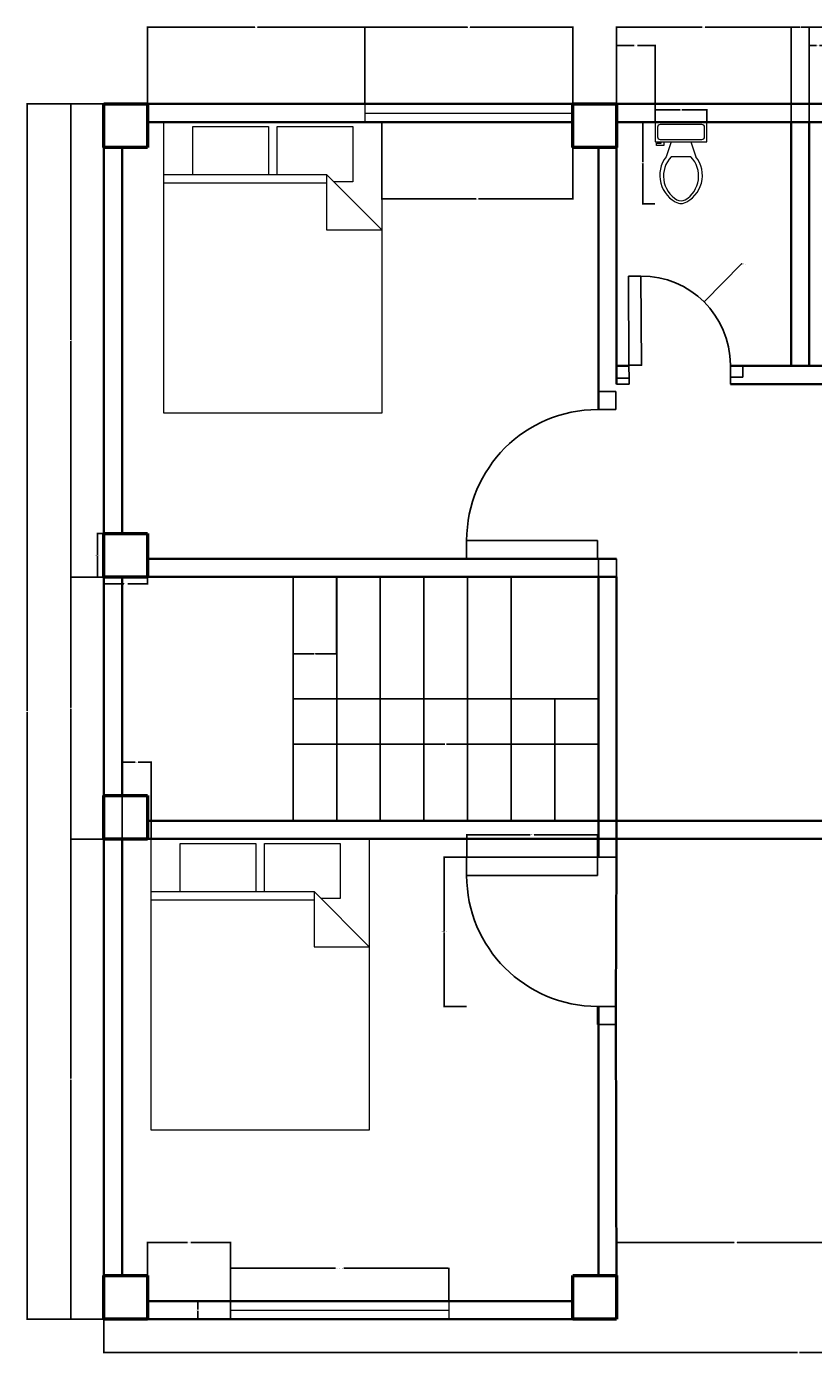
# Model space of a CAD drawing. Units: inches. Extents: x 2082 to 2506, y 790 to 1201.
# Tile 1 of 3: x 2082 to 2298, y 836 to 1201. Entities that reach past the tile are written whole.
import ezdxf

# ---------------------------------------------------------------- set-up
doc = ezdxf.new("R2010")
doc.units = ezdxf.units.IN
for name, color, linetype, lineweight in [('A-ANNO-DIMS', 2, 'Continuous', 18), ('A-COLS', 7, 'Continuous', 50), ('A-DOOR', 3, 'Continuous', 25), ('A-FLOR-FIXT', 9, 'Continuous', 18), ('A-FLOR-STRS', 2, 'Continuous', 25), ('A-FURN', 8, 'Continuous', 18), ('A-GLAZ', 4, 'Continuous', 18), ('A-WALL', 7, 'Continuous', 35)]:
    doc.layers.add(name, color=color, linetype=linetype, lineweight=lineweight)
doc.styles.get("Standard").update_dxf_attribs({"font": 'arial.ttf'})
doc.dimstyles.get("Standard").update_dxf_attribs({"dimtxt": 0.18, "dimasz": 0.18, "dimexe": 0.18, "dimexo": 0.0625, "dimgap": 0.09, "dimtad": 0, "dimtih": 1, "dimtoh": 1, "dimdec": 4, "dimzin": 0, "dimdsep": 46, "dimlunit": 4, "dimtxsty": 'Standard', "dimcen": 0.09, "dimadec": 0, "dimazin": 0, "dimtfac": 1, "dimtdec": 4, "dimtofl": 0, "dimtmove": 0, "dimatfit": 3, "dimfxl": 1, "dimtolj": 1, "dimtzin": 0, "dimarcsym": 0})

# ---------------------------------------------------------------- blocks, each defined once
blk = doc.blocks.new('Toilet - top')
for p, q in [((9.5, -6), (9.5, -2)), ((-10, -8.5), (-8, -8.5)), ((-10, -9.5), (-10, -8.5)), ((-7, -9.5), (-10, -9.5)), ((-8, -8.5), (-8, -8)), ((-7, -8), (-7, -9.5)), ((-4, -8), (-6, -14)), ((4, -8), (6, -14)), ((4, -14), (-4, -14))]:
    blk.add_line(p, q)
blk.add_lwpolyline([(10.5, -8), (10.5, 0), (-10.5, 0), (-10.5, -8)], close=True)
for points in [[(-9.5, -2), (-9.5, -6)], [(8.5, -1), (-8.5, -1)], [(-8.5, -7), (8.5, -7)]]:
    blk.add_lwpolyline(points)
for centre, radius, start, end in [((-8.62, -1.88), 0.884, 81.8699, 188.1301), ((8.62, -1.88), 0.884, 351.8699, 98.1301), ((-8.62, -6.12), 0.884, 171.8699, 278.1301), ((8.62, -6.12), 0.884, 261.8699, 8.1301), ((3.52, -21.58), 12.17, 141.4691, 247.9714), ((4.2, -21.82), 11.33, 136.3677, 238.9468), ((-3.52, -21.58), 12.17, 292.0284, 38.5307), ((-4.2, -21.82), 11.33, 301.053, 43.6321), ((0, -27.88), 4, 245.7318, 294.2682), ((0, -29), 4, 254.8605, 285.1395)]:
    blk.add_arc(centre, radius, start, end)
blk = doc.blocks.new('Bed - Queen')
for p, q in [((0, -80.00003), (0, 0)), ((0, 0), (59.99999, 0)), ((59.99999, 0), (59.99999, -80.00003)), ((7.99999, -1.2), (28.79998, -1.2)), ((7.99999, -14.4), (7.99999, -1.2)), ((28.79998, -1.2), (28.79998, -14.4)), ((31.19999, -1.2), (51.99999, -1.2)), ((31.19999, -14.4), (31.19999, -1.2)), ((51.99999, -1.2), (51.99999, -16.4)), ((0, -14.4), (44.8, -14.4)), ((59.99999, -29.6), (44.8, -14.4)), ((44.8, -14.4), (44.8, -29.6)), ((44.8, -16.8), (0, -16.8)), ((51.99999, -16.4), (46.79936, -16.4)), ((44.8, -29.6), (59.99999, -29.6)), ((59.99999, -80.00003), (0, -80.00003))]:
    blk.add_line(p, q)
blk = doc.blocks.new('DOOR-SWING-36IN')
for p, q in [((0, 0), (0, 5)), ((0, 5), (36, 5)), ((36, 5), (36, 0)), ((36, 0), (0, 0))]:
    blk.add_line(p, q)
blk.add_arc((0, 5), 36, 0, 90)
blk = doc.blocks.new('WIN-60IN')
for p, q in [((0, 5), (12, 5)), ((0, 5), (0, 0)), ((12, 5), (60, 5)), ((60, 5), (60, 0)), ((0, 2.5), (60, 2.5)), ((0, 0), (60, 0))]:
    blk.add_line(p, q)
blk = doc.blocks.new('COL-12X12IN')
for p, q in [((0, 12), (12, 12)), ((0, 0), (0, 12)), ((12, 12), (12, 0)), ((12, 0), (0, 0))]:
    blk.add_line(p, q)
blk = doc.blocks.new('*D8')
at = {"layer": 'A-ANNO-DIMS', "color": 0, "lineweight": -2, "transparency": 16777216}
for p, q in [((2102.86, 1061.45), (2100.94, 1061.45)), ((2101.12, 1061.27), (2101.12, 1055.63)), ((2101.12, 1049.63), (2101.12, 1055.27)), ((2102.86, 1049.45), (2100.94, 1049.45))]:
    blk.add_line(p, q, dxfattribs=at)
at = {"layer": 'A-ANNO-DIMS', "color": 0, "transparency": 16777216}
for points in [[(2101.09, 1061.27), (2101.15, 1061.27), (2101.12, 1061.45)], [(2101.09, 1049.63), (2101.15, 1049.63), (2101.12, 1049.45)]]:
    blk.add_solid(points, dxfattribs=at)
at = {"layer": 'Defpoints', "color": 0, "transparency": 16777216}
for p in [(2101.12, 1061.45), (2102.92, 1061.45), (2102.92, 1049.45)]:
    blk.add_point(p, dxfattribs=at)
at = {"layer": 'A-ANNO-DIMS', "color": 0, "transparency": 16777216, "insert": (2101.12, 1055.45), "char_height": 0.18, "attachment_point": 5}
blk.add_mtext('\\A1;COLUMN 12 TYP.', dxfattribs=at)
blk = doc.blocks.new('*D9')
at = {"layer": 'A-ANNO-DIMS', "color": 0, "lineweight": -2, "transparency": 16777216}
for p, q in [((2102.92, 1049.39), (2102.92, 1047.47)), ((2103.1, 1047.65), (2108.4, 1047.65)), ((2114.74, 1047.65), (2109.44, 1047.65)), ((2114.92, 1049.39), (2114.92, 1047.47))]:
    blk.add_line(p, q, dxfattribs=at)
at = {"layer": 'A-ANNO-DIMS', "color": 0, "transparency": 16777216}
for points in [[(2103.1, 1047.68), (2103.1, 1047.62), (2102.92, 1047.65)], [(2114.74, 1047.68), (2114.74, 1047.62), (2114.92, 1047.65)]]:
    blk.add_solid(points, dxfattribs=at)
at = {"layer": 'Defpoints', "color": 0, "transparency": 16777216}
for p in [(2102.92, 1049.45), (2102.92, 1047.65), (2114.92, 1049.45)]:
    blk.add_point(p, dxfattribs=at)
at = {"layer": 'A-ANNO-DIMS', "color": 0, "transparency": 16777216, "insert": (2108.92, 1047.65), "char_height": 0.18, "attachment_point": 5}
blk.add_mtext('\\A1;12 TYP.', dxfattribs=at)
blk = doc.blocks.new('*D12')
at = {"layer": 'A-ANNO-DIMS', "color": 0, "lineweight": -2, "transparency": 16777216}
for p, q in [((2137.75, 850.56), (2137.75, 859.68)), ((2137.93, 859.5), (2166.63, 859.5)), ((2197.57, 859.5), (2168.87, 859.5)), ((2197.75, 850.56), (2197.75, 859.68))]:
    blk.add_line(p, q, dxfattribs=at)
at = {"layer": 'A-ANNO-DIMS', "color": 0, "transparency": 16777216}
for points in [[(2137.93, 859.53), (2137.93, 859.47), (2137.75, 859.5)], [(2197.57, 859.53), (2197.57, 859.47), (2197.75, 859.5)]]:
    blk.add_solid(points, dxfattribs=at)
at = {"layer": 'Defpoints', "color": 0, "transparency": 16777216}
for p in [(2197.75, 859.5), (2137.75, 850.5), (2197.75, 850.5)]:
    blk.add_point(p, dxfattribs=at)
at = {"layer": 'A-ANNO-DIMS', "color": 0, "transparency": 16777216, "insert": (2167.75, 859.5), "char_height": 0.18, "attachment_point": 5}
blk.add_mtext('\\A1;WINDOW 60 TYP.', dxfattribs=at)
blk = doc.blocks.new('*D13')
at = {"layer": 'A-ANNO-DIMS', "color": 0, "lineweight": -2, "transparency": 16777216}
for p, q in [((2137.69, 850.5), (2128.57, 850.5)), ((2128.75, 850.32), (2128.75, 848.18)), ((2128.75, 845.68), (2128.75, 847.82)), ((2137.69, 845.5), (2128.57, 845.5))]:
    blk.add_line(p, q, dxfattribs=at)
at = {"layer": 'A-ANNO-DIMS', "color": 0, "transparency": 16777216}
for points in [[(2128.72, 850.32), (2128.78, 850.32), (2128.75, 850.5)], [(2128.72, 845.68), (2128.78, 845.68), (2128.75, 845.5)]]:
    blk.add_solid(points, dxfattribs=at)
at = {"layer": 'Defpoints', "color": 0, "transparency": 16777216}
for p in [(2128.75, 850.5), (2137.75, 850.5), (2137.75, 845.5)]:
    blk.add_point(p, dxfattribs=at)
at = {"layer": 'A-ANNO-DIMS', "color": 0, "transparency": 16777216, "insert": (2128.75, 848), "char_height": 0.18, "attachment_point": 5}
blk.add_mtext('\\A1;5 TYP.', dxfattribs=at)
blk = doc.blocks.new('*D14')
at = {"layer": 'A-ANNO-DIMS', "color": 0, "lineweight": -2, "transparency": 16777216}
for p, q in [((2202.61, 972.5), (2196.35, 972.5)), ((2196.53, 972.32), (2196.53, 952.18)), ((2196.53, 931.68), (2196.53, 951.82)), ((2202.61, 931.5), (2196.35, 931.5))]:
    blk.add_line(p, q, dxfattribs=at)
at = {"layer": 'A-ANNO-DIMS', "color": 0, "transparency": 16777216}
for points in [[(2196.5, 972.32), (2196.56, 972.32), (2196.53, 972.5)], [(2196.5, 931.68), (2196.56, 931.68), (2196.53, 931.5)]]:
    blk.add_solid(points, dxfattribs=at)
at = {"layer": 'Defpoints', "color": 0, "transparency": 16777216}
for p in [(2202.68, 972.5), (2196.53, 931.5), (2202.68, 931.5)]:
    blk.add_point(p, dxfattribs=at)
at = {"layer": 'A-ANNO-DIMS', "color": 0, "transparency": 16777216, "insert": (2196.53, 952), "char_height": 0.18, "attachment_point": 5}
blk.add_mtext('\\A1;DOOR 41 TYP.', dxfattribs=at)
blk = doc.blocks.new('*D15')
at = {"layer": 'A-ANNO-DIMS', "color": 0, "lineweight": -2, "transparency": 16777216}
for p, q in [((2202.68, 972.56), (2202.68, 978.83)), ((2202.86, 978.65), (2220.15, 978.65)), ((2238.5, 978.65), (2221.2, 978.65)), ((2238.68, 972.56), (2238.68, 978.83))]:
    blk.add_line(p, q, dxfattribs=at)
at = {"layer": 'A-ANNO-DIMS', "color": 0, "transparency": 16777216}
for points in [[(2202.86, 978.68), (2202.86, 978.62), (2202.68, 978.65)], [(2238.5, 978.68), (2238.5, 978.62), (2238.68, 978.65)]]:
    blk.add_solid(points, dxfattribs=at)
at = {"layer": 'Defpoints', "color": 0, "transparency": 16777216}
for p in [(2202.68, 978.65), (2202.68, 972.5), (2238.68, 972.5)]:
    blk.add_point(p, dxfattribs=at)
at = {"layer": 'A-ANNO-DIMS', "color": 0, "transparency": 16777216, "insert": (2220.68, 978.65), "char_height": 0.18, "attachment_point": 5}
blk.add_mtext('\\A1;36 TYP.', dxfattribs=at)
blk = doc.blocks.new('*D16')
at = {"layer": 'A-ANNO-DIMS', "color": 0, "lineweight": -2, "transparency": 16777216}
for p, q in [((2254.46, 1174.5), (2250.98, 1174.5)), ((2251.16, 1174.32), (2251.16, 1163.48)), ((2251.16, 1152.27), (2251.16, 1163.11)), ((2254.46, 1152.09), (2250.98, 1152.09))]:
    blk.add_line(p, q, dxfattribs=at)
at = {"layer": 'A-ANNO-DIMS', "color": 0, "transparency": 16777216}
for points in [[(2251.13, 1174.32), (2251.19, 1174.32), (2251.16, 1174.5)], [(2251.13, 1152.27), (2251.19, 1152.27), (2251.16, 1152.09)]]:
    blk.add_solid(points, dxfattribs=at)
at = {"layer": 'Defpoints', "color": 0, "transparency": 16777216}
for p in [(2251.16, 1174.5), (2254.52, 1174.5), (2254.52, 1152.09)]:
    blk.add_point(p, dxfattribs=at)
at = {"layer": 'A-ANNO-DIMS', "color": 0, "transparency": 16777216, "insert": (2251.16, 1163.3), "char_height": 0.18, "attachment_point": 5}
blk.add_mtext('\\A1;WC 22', dxfattribs=at)
blk = doc.blocks.new('*D17')
at = {"layer": 'A-ANNO-DIMS', "color": 0, "lineweight": -2, "transparency": 16777216}
for p, q in [((2254.52, 1174.56), (2254.52, 1178.04)), ((2268.76, 1174.56), (2268.76, 1178.04)), ((2254.7, 1177.86), (2261.43, 1177.86)), ((2268.58, 1177.86), (2261.85, 1177.86))]:
    blk.add_line(p, q, dxfattribs=at)
at = {"layer": 'A-ANNO-DIMS', "color": 0, "transparency": 16777216}
for points in [[(2254.7, 1177.89), (2254.7, 1177.83), (2254.52, 1177.86)], [(2268.58, 1177.89), (2268.58, 1177.83), (2268.76, 1177.86)]]:
    blk.add_solid(points, dxfattribs=at)
at = {"layer": 'Defpoints', "color": 0, "transparency": 16777216}
for p in [(2254.52, 1174.5), (2268.76, 1177.86), (2268.76, 1174.5)]:
    blk.add_point(p, dxfattribs=at)
at = {"layer": 'A-ANNO-DIMS', "color": 0, "transparency": 16777216, "insert": (2261.64, 1177.86), "char_height": 0.18, "attachment_point": 5}
blk.add_mtext('\\A1;14', dxfattribs=at)
blk = doc.blocks.new('*D24')
at = {"layer": 'A-ANNO-DIMS', "color": 0, "lineweight": -2, "transparency": 16777216}
for p, q in [((2102.92, 857.43), (2102.92, 836.21)), ((2484.95, 857.32), (2484.95, 836.1)), ((2103.1, 836.39), (2293.64, 836.34)), ((2484.77, 836.28), (2294.22, 836.34))]:
    blk.add_line(p, q, dxfattribs=at)
at = {"layer": 'A-ANNO-DIMS', "color": 0, "transparency": 16777216}
for points in [[(2103.1, 836.42), (2103.1, 836.36), (2102.92, 836.39)], [(2484.77, 836.31), (2484.77, 836.25), (2484.95, 836.28)]]:
    blk.add_solid(points, dxfattribs=at)
at = {"layer": 'Defpoints', "color": 0, "transparency": 16777216}
for p in [(2102.92, 857.49), (2484.95, 857.38), (2102.92, 836.39)]:
    blk.add_point(p, dxfattribs=at)
at = {"layer": 'A-ANNO-DIMS', "color": 0, "transparency": 16777216, "insert": (2293.93, 836.34), "char_height": 0.18, "attachment_point": 5}
blk.add_mtext('\\A1;382', dxfattribs=at)
blk = doc.blocks.new('*D25')
at = {"layer": 'A-ANNO-DIMS', "color": 0, "lineweight": -2, "transparency": 16777216}
for p, q in [((2102.86, 1179.5), (2081.64, 1179.5)), ((2081.82, 1179.32), (2081.82, 1012.68)), ((2081.82, 845.67), (2081.82, 1012.31)), ((2102.86, 845.49), (2081.64, 845.49))]:
    blk.add_line(p, q, dxfattribs=at)
at = {"layer": 'A-ANNO-DIMS', "color": 0, "transparency": 16777216}
for points in [[(2081.79, 1179.32), (2081.85, 1179.32), (2081.82, 1179.5)], [(2081.79, 845.67), (2081.85, 845.67), (2081.82, 845.49)]]:
    blk.add_solid(points, dxfattribs=at)
at = {"layer": 'Defpoints', "color": 0, "transparency": 16777216}
for p in [(2081.82, 1179.5), (2102.92, 1179.5), (2102.92, 845.49)]:
    blk.add_point(p, dxfattribs=at)
at = {"layer": 'A-ANNO-DIMS', "color": 0, "transparency": 16777216, "insert": (2081.82, 1012.5), "char_height": 0.18, "attachment_point": 5}
blk.add_mtext('\\A1;334', dxfattribs=at)
blk = doc.blocks.new('*D26')
at = {"layer": 'A-ANNO-DIMS', "color": 0, "lineweight": -2, "transparency": 16777216}
for p, q in [((2114.86, 977.48), (2093.64, 977.48)), ((2093.82, 977.3), (2093.82, 911.67)), ((2093.82, 845.67), (2093.82, 911.3)), ((2114.86, 845.49), (2093.64, 845.49))]:
    blk.add_line(p, q, dxfattribs=at)
at = {"layer": 'A-ANNO-DIMS', "color": 0, "transparency": 16777216}
for points in [[(2093.79, 977.3), (2093.85, 977.3), (2093.82, 977.48)], [(2093.79, 845.67), (2093.85, 845.67), (2093.82, 845.49)]]:
    blk.add_solid(points, dxfattribs=at)
at = {"layer": 'Defpoints', "color": 0, "transparency": 16777216}
for p in [(2093.82, 977.48), (2114.92, 977.48), (2114.92, 845.49)]:
    blk.add_point(p, dxfattribs=at)
at = {"layer": 'A-ANNO-DIMS', "color": 0, "transparency": 16777216, "insert": (2093.82, 911.49), "char_height": 0.18, "attachment_point": 5}
blk.add_mtext('\\A1;132', dxfattribs=at)
blk = doc.blocks.new('*D27')
at = {"layer": 'A-ANNO-DIMS', "color": 0, "lineweight": -2, "transparency": 16777216}
for p, q in [((2114.86, 1049.45), (2093.64, 1049.45)), ((2093.82, 1049.27), (2093.82, 1013.65)), ((2093.82, 977.66), (2093.82, 1013.28)), ((2114.86, 977.48), (2093.64, 977.48))]:
    blk.add_line(p, q, dxfattribs=at)
at = {"layer": 'A-ANNO-DIMS', "color": 0, "transparency": 16777216}
for points in [[(2093.79, 1049.27), (2093.85, 1049.27), (2093.82, 1049.45)], [(2093.79, 977.66), (2093.85, 977.66), (2093.82, 977.48)]]:
    blk.add_solid(points, dxfattribs=at)
at = {"layer": 'Defpoints', "color": 0, "transparency": 16777216}
for p in [(2093.82, 1049.45), (2114.92, 1049.45), (2114.92, 977.48)]:
    blk.add_point(p, dxfattribs=at)
at = {"layer": 'A-ANNO-DIMS', "color": 0, "transparency": 16777216, "insert": (2093.82, 1013.47), "char_height": 0.18, "attachment_point": 5}
blk.add_mtext('\\A1;71.97', dxfattribs=at)
blk = doc.blocks.new('*D28')
at = {"layer": 'A-ANNO-DIMS', "color": 0, "lineweight": -2, "transparency": 16777216}
for p, q in [((2114.86, 1179.5), (2093.64, 1179.5)), ((2093.82, 1179.32), (2093.82, 1114.66)), ((2093.82, 1049.63), (2093.82, 1114.29)), ((2114.86, 1049.45), (2093.64, 1049.45))]:
    blk.add_line(p, q, dxfattribs=at)
at = {"layer": 'A-ANNO-DIMS', "color": 0, "transparency": 16777216}
for points in [[(2093.79, 1179.32), (2093.85, 1179.32), (2093.82, 1179.5)], [(2093.79, 1049.63), (2093.85, 1049.63), (2093.82, 1049.45)]]:
    blk.add_solid(points, dxfattribs=at)
at = {"layer": 'Defpoints', "color": 0, "transparency": 16777216}
for p in [(2093.82, 1179.5), (2114.92, 1179.5), (2114.92, 1049.45)]:
    blk.add_point(p, dxfattribs=at)
at = {"layer": 'A-ANNO-DIMS', "color": 0, "transparency": 16777216, "insert": (2093.82, 1114.47), "char_height": 0.18, "attachment_point": 5}
blk.add_mtext('\\A1;130.05', dxfattribs=at)
blk = doc.blocks.new('*D29')
at = {"layer": 'A-ANNO-DIMS', "color": 0, "lineweight": -2, "transparency": 16777216}
for p, q in [((2114.92, 1179.56), (2114.92, 1200.78)), ((2115.1, 1200.6), (2144.4, 1200.6)), ((2174.49, 1200.6), (2145.19, 1200.6)), ((2174.67, 1179.56), (2174.67, 1200.78))]:
    blk.add_line(p, q, dxfattribs=at)
at = {"layer": 'A-ANNO-DIMS', "color": 0, "transparency": 16777216}
for points in [[(2115.1, 1200.63), (2115.1, 1200.57), (2114.92, 1200.6)], [(2174.49, 1200.63), (2174.49, 1200.57), (2174.67, 1200.6)]]:
    blk.add_solid(points, dxfattribs=at)
at = {"layer": 'Defpoints', "color": 0, "transparency": 16777216}
for p in [(2174.67, 1200.6), (2114.92, 1179.5), (2174.67, 1179.5)]:
    blk.add_point(p, dxfattribs=at)
at = {"layer": 'A-ANNO-DIMS', "color": 0, "transparency": 16777216, "insert": (2144.8, 1200.6), "char_height": 0.18, "attachment_point": 5}
blk.add_mtext('\\A1;59.75', dxfattribs=at)
blk = doc.blocks.new('*D30')
at = {"layer": 'A-ANNO-DIMS', "color": 0, "lineweight": -2, "transparency": 16777216}
for p, q in [((2174.67, 1179.56), (2174.67, 1200.78)), ((2174.85, 1200.6), (2202.87, 1200.6)), ((2231.68, 1200.6), (2203.66, 1200.6)), ((2231.86, 1179.56), (2231.86, 1200.78))]:
    blk.add_line(p, q, dxfattribs=at)
at = {"layer": 'A-ANNO-DIMS', "color": 0, "transparency": 16777216}
for points in [[(2174.85, 1200.63), (2174.85, 1200.57), (2174.67, 1200.6)], [(2231.68, 1200.63), (2231.68, 1200.57), (2231.86, 1200.6)]]:
    blk.add_solid(points, dxfattribs=at)
at = {"layer": 'Defpoints', "color": 0, "transparency": 16777216}
for p in [(2231.86, 1200.6), (2174.67, 1179.5), (2231.86, 1179.5)]:
    blk.add_point(p, dxfattribs=at)
at = {"layer": 'A-ANNO-DIMS', "color": 0, "transparency": 16777216, "insert": (2203.26, 1200.6), "char_height": 0.18, "attachment_point": 5}
blk.add_mtext('\\A1;57.18', dxfattribs=at)
blk = doc.blocks.new('*D31')
at = {"layer": 'A-ANNO-DIMS', "color": 0, "lineweight": -2, "transparency": 16777216}
for p, q in [((2243.86, 1174.56), (2243.86, 1200.78)), ((2244.04, 1200.6), (2267.49, 1200.6)), ((2291.74, 1200.6), (2268.29, 1200.6)), ((2291.92, 1174.56), (2291.92, 1200.78))]:
    blk.add_line(p, q, dxfattribs=at)
at = {"layer": 'A-ANNO-DIMS', "color": 0, "transparency": 16777216}
for points in [[(2244.04, 1200.63), (2244.04, 1200.57), (2243.86, 1200.6)], [(2291.74, 1200.63), (2291.74, 1200.57), (2291.92, 1200.6)]]:
    blk.add_solid(points, dxfattribs=at)
at = {"layer": 'Defpoints', "color": 0, "transparency": 16777216}
for p in [(2291.92, 1200.6), (2243.86, 1174.5), (2291.92, 1174.5)]:
    blk.add_point(p, dxfattribs=at)
at = {"layer": 'A-ANNO-DIMS', "color": 0, "transparency": 16777216, "insert": (2267.89, 1200.6), "char_height": 0.18, "attachment_point": 5}
blk.add_mtext('\\A1;48.07', dxfattribs=at)
blk = doc.blocks.new('*D32')
at = {"layer": 'A-ANNO-DIMS', "color": 0, "lineweight": -2, "transparency": 16777216}
for p, q in [((2291.92, 1174.56), (2291.92, 1200.78)), ((2292.1, 1200.6), (2294.27, 1200.6)), ((2296.74, 1200.6), (2294.57, 1200.6)), ((2296.92, 1174.56), (2296.92, 1200.78))]:
    blk.add_line(p, q, dxfattribs=at)
at = {"layer": 'A-ANNO-DIMS', "color": 0, "transparency": 16777216}
for points in [[(2292.1, 1200.63), (2292.1, 1200.57), (2291.92, 1200.6)], [(2296.74, 1200.63), (2296.74, 1200.57), (2296.92, 1200.6)]]:
    blk.add_solid(points, dxfattribs=at)
at = {"layer": 'Defpoints', "color": 0, "transparency": 16777216}
for p in [(2296.92, 1200.6), (2291.92, 1174.5), (2296.92, 1174.5)]:
    blk.add_point(p, dxfattribs=at)
at = {"layer": 'A-ANNO-DIMS', "color": 0, "transparency": 16777216, "insert": (2294.42, 1200.6), "char_height": 0.18, "attachment_point": 5}
blk.add_mtext('\\A1;5', dxfattribs=at)
blk = doc.blocks.new('*D33')
at = {"layer": 'A-ANNO-DIMS', "color": 0, "lineweight": -2, "transparency": 16777216}
for p, q in [((2296.92, 1174.56), (2296.92, 1200.78)), ((2297.1, 1200.6), (2317.7, 1200.6)), ((2338.74, 1200.6), (2318.15, 1200.6)), ((2338.92, 1174.56), (2338.92, 1200.78))]:
    blk.add_line(p, q, dxfattribs=at)
at = {"layer": 'A-ANNO-DIMS', "color": 0, "transparency": 16777216}
for points in [[(2297.1, 1200.63), (2297.1, 1200.57), (2296.92, 1200.6)], [(2338.74, 1200.63), (2338.74, 1200.57), (2338.92, 1200.6)]]:
    blk.add_solid(points, dxfattribs=at)
at = {"layer": 'Defpoints', "color": 0, "transparency": 16777216}
for p in [(2338.92, 1200.6), (2296.92, 1174.5), (2338.92, 1174.5)]:
    blk.add_point(p, dxfattribs=at)
at = {"layer": 'A-ANNO-DIMS', "color": 0, "transparency": 16777216, "insert": (2317.92, 1200.6), "char_height": 0.18, "attachment_point": 5}
blk.add_mtext('\\A1;42', dxfattribs=at)
blk = doc.blocks.new('*D39')
at = {"layer": 'A-ANNO-DIMS', "color": 0, "lineweight": -2, "transparency": 16777216}
for p, q in [((2154.92, 982.56), (2154.92, 1003.78)), ((2155.1, 1003.6), (2196.7, 1003.6)), ((2238.74, 1003.6), (2197.14, 1003.6)), ((2238.92, 982.56), (2238.92, 1003.78))]:
    blk.add_line(p, q, dxfattribs=at)
at = {"layer": 'A-ANNO-DIMS', "color": 0, "transparency": 16777216}
for points in [[(2155.1, 1003.63), (2155.1, 1003.57), (2154.92, 1003.6)], [(2238.74, 1003.63), (2238.74, 1003.57), (2238.92, 1003.6)]]:
    blk.add_solid(points, dxfattribs=at)
at = {"layer": 'Defpoints', "color": 0, "transparency": 16777216}
for p in [(2238.92, 1003.6), (2154.92, 982.5), (2238.92, 982.5)]:
    blk.add_point(p, dxfattribs=at)
at = {"layer": 'A-ANNO-DIMS', "color": 0, "transparency": 16777216, "insert": (2196.92, 1003.6), "char_height": 0.18, "attachment_point": 5}
blk.add_mtext('\\A1;84', dxfattribs=at)
blk = doc.blocks.new('*D40')
at = {"layer": 'A-ANNO-DIMS', "color": 0, "lineweight": -2, "transparency": 16777216}
for p, q in [((2154.92, 1049.44), (2154.92, 1028.22)), ((2166.92, 1049.44), (2166.92, 1028.22)), ((2155.1, 1028.4), (2160.71, 1028.4)), ((2166.74, 1028.4), (2161.13, 1028.4))]:
    blk.add_line(p, q, dxfattribs=at)
at = {"layer": 'A-ANNO-DIMS', "color": 0, "transparency": 16777216}
for points in [[(2155.1, 1028.43), (2155.1, 1028.37), (2154.92, 1028.4)], [(2166.74, 1028.43), (2166.74, 1028.37), (2166.92, 1028.4)]]:
    blk.add_solid(points, dxfattribs=at)
at = {"layer": 'Defpoints', "color": 0, "transparency": 16777216}
for p in [(2154.92, 1049.5), (2166.92, 1049.5), (2154.92, 1028.4)]:
    blk.add_point(p, dxfattribs=at)
at = {"layer": 'A-ANNO-DIMS', "color": 0, "transparency": 16777216, "insert": (2160.92, 1028.4), "char_height": 0.18, "attachment_point": 5}
blk.add_mtext('\\A1;12', dxfattribs=at)
blk = doc.blocks.new('*D41')
at = {"layer": 'A-ANNO-DIMS', "color": 0, "lineweight": -2, "transparency": 16777216}
for p, q in [((2243.9, 845.56), (2243.9, 866.78)), ((2244.08, 866.6), (2276.28, 866.6)), ((2309.24, 866.6), (2277.04, 866.6)), ((2309.42, 845.56), (2309.42, 866.78))]:
    blk.add_line(p, q, dxfattribs=at)
at = {"layer": 'A-ANNO-DIMS', "color": 0, "transparency": 16777216}
for points in [[(2244.08, 866.63), (2244.08, 866.57), (2243.9, 866.6)], [(2309.24, 866.63), (2309.24, 866.57), (2309.42, 866.6)]]:
    blk.add_solid(points, dxfattribs=at)
at = {"layer": 'Defpoints', "color": 0, "transparency": 16777216}
for p in [(2309.42, 866.6), (2243.9, 845.5), (2309.42, 845.5)]:
    blk.add_point(p, dxfattribs=at)
at = {"layer": 'A-ANNO-DIMS', "color": 0, "transparency": 16777216, "insert": (2276.66, 866.6), "char_height": 0.18, "attachment_point": 5}
blk.add_mtext('\\A1;65.51', dxfattribs=at)
blk = doc.blocks.new('*D42')
at = {"layer": 'A-ANNO-DIMS', "color": 0, "lineweight": -2, "transparency": 16777216}
for p, q in [((2114.92, 845.55), (2114.92, 866.77)), ((2115.1, 866.59), (2125.86, 866.6)), ((2137.56, 866.6), (2126.8, 866.6)), ((2137.75, 845.56), (2137.74, 866.78))]:
    blk.add_line(p, q, dxfattribs=at)
at = {"layer": 'A-ANNO-DIMS', "color": 0, "transparency": 16777216}
for points in [[(2115.1, 866.62), (2115.1, 866.56), (2114.92, 866.59)], [(2137.56, 866.63), (2137.56, 866.57), (2137.74, 866.6)]]:
    blk.add_solid(points, dxfattribs=at)
at = {"layer": 'Defpoints', "color": 0, "transparency": 16777216}
for p in [(2137.74, 866.6), (2114.92, 845.49), (2137.75, 845.5)]:
    blk.add_point(p, dxfattribs=at)
at = {"layer": 'A-ANNO-DIMS', "color": 0, "transparency": 16777216, "insert": (2126.33, 866.6), "char_height": 0.18, "attachment_point": 5}
blk.add_mtext('\\A1;22.825', dxfattribs=at)
blk = doc.blocks.new('*D49')
at = {"layer": 'A-ANNO-DIMS', "color": 0, "lineweight": -2, "transparency": 16777216}
for p, q in [((2179.35, 1174.44), (2179.35, 1153.22)), ((2231.86, 1174.44), (2231.86, 1153.22)), ((2179.53, 1153.4), (2205.28, 1153.4)), ((2231.68, 1153.4), (2205.93, 1153.4))]:
    blk.add_line(p, q, dxfattribs=at)
at = {"layer": 'A-ANNO-DIMS', "color": 0, "transparency": 16777216}
for points in [[(2179.53, 1153.43), (2179.53, 1153.37), (2179.35, 1153.4)], [(2231.68, 1153.43), (2231.68, 1153.37), (2231.86, 1153.4)]]:
    blk.add_solid(points, dxfattribs=at)
at = {"layer": 'Defpoints', "color": 0, "transparency": 16777216}
for p in [(2179.35, 1174.5), (2231.86, 1174.5), (2179.35, 1153.4)]:
    blk.add_point(p, dxfattribs=at)
at = {"layer": 'A-ANNO-DIMS', "color": 0, "transparency": 16777216, "insert": (2205.6, 1153.4), "char_height": 0.18, "attachment_point": 5}
blk.add_mtext('\\A1;52.5', dxfattribs=at)
blk = doc.blocks.new('*D51')
at = {"layer": 'A-ANNO-DIMS', "color": 0, "lineweight": -2, "transparency": 16777216}
for p, q in [((2107.92, 977.56), (2107.92, 998.78)), ((2108.1, 998.6), (2111.52, 998.6)), ((2115.73, 998.6), (2112.31, 998.6)), ((2115.91, 977.56), (2115.91, 998.78))]:
    blk.add_line(p, q, dxfattribs=at)
at = {"layer": 'A-ANNO-DIMS', "color": 0, "transparency": 16777216}
for points in [[(2108.1, 998.63), (2108.1, 998.57), (2107.92, 998.6)], [(2115.73, 998.63), (2115.73, 998.57), (2115.91, 998.6)]]:
    blk.add_solid(points, dxfattribs=at)
at = {"layer": 'Defpoints', "color": 0, "transparency": 16777216}
for p in [(2115.91, 998.6), (2107.92, 977.5), (2115.91, 977.5)]:
    blk.add_point(p, dxfattribs=at)
at = {"layer": 'A-ANNO-DIMS', "color": 0, "transparency": 16777216, "insert": (2111.91, 998.6), "char_height": 0.18, "attachment_point": 5}
blk.add_mtext('\\A1;7.982', dxfattribs=at)
blk = doc.blocks.new('*D52')
at = {"layer": 'A-ANNO-DIMS', "color": 0, "lineweight": -2, "transparency": 16777216}
for p, q in [((2243.86, 1174.56), (2243.86, 1195.78)), ((2244.04, 1195.6), (2248.73, 1195.6)), ((2254.34, 1195.6), (2249.64, 1195.6)), ((2254.52, 1174.56), (2254.52, 1195.78))]:
    blk.add_line(p, q, dxfattribs=at)
at = {"layer": 'A-ANNO-DIMS', "color": 0, "transparency": 16777216}
for points in [[(2244.04, 1195.63), (2244.04, 1195.57), (2243.86, 1195.6)], [(2254.34, 1195.63), (2254.34, 1195.57), (2254.52, 1195.6)]]:
    blk.add_solid(points, dxfattribs=at)
at = {"layer": 'Defpoints', "color": 0, "transparency": 16777216}
for p in [(2254.52, 1195.6), (2243.86, 1174.5), (2254.52, 1174.5)]:
    blk.add_point(p, dxfattribs=at)
at = {"layer": 'A-ANNO-DIMS', "color": 0, "transparency": 16777216, "insert": (2249.19, 1195.6), "char_height": 0.18, "attachment_point": 5}
blk.add_mtext('\\A1;10.666', dxfattribs=at)
blk = doc.blocks.new('*D53')
at = {"layer": 'A-ANNO-DIMS', "color": 0, "lineweight": -2, "transparency": 16777216}
for p, q in [((2296.92, 1174.56), (2296.92, 1195.78)), ((2297.1, 1195.6), (2298.93, 1195.6)), ((2301.55, 1195.6), (2299.72, 1195.6)), ((2301.73, 1174.56), (2301.73, 1195.78))]:
    blk.add_line(p, q, dxfattribs=at)
at = {"layer": 'A-ANNO-DIMS', "color": 0, "transparency": 16777216}
for points in [[(2297.1, 1195.63), (2297.1, 1195.57), (2296.92, 1195.6)], [(2301.55, 1195.63), (2301.55, 1195.57), (2301.73, 1195.6)]]:
    blk.add_solid(points, dxfattribs=at)
at = {"layer": 'Defpoints', "color": 0, "transparency": 16777216}
for p in [(2301.73, 1195.6), (2296.92, 1174.5), (2301.73, 1174.5)]:
    blk.add_point(p, dxfattribs=at)
at = {"layer": 'A-ANNO-DIMS', "color": 0, "transparency": 16777216, "insert": (2299.33, 1195.6), "char_height": 0.18, "attachment_point": 5}
blk.add_mtext('\\A1;4.805', dxfattribs=at)
blk = doc.blocks.new('*D56')
at = {"layer": 'A-ANNO-DIMS', "color": 0, "lineweight": -2, "transparency": 16777216}
for p, q in [((2278.3, 1135.55), (2268.09, 1125.23)), ((2278.48, 1135.55), (2278.3, 1135.55)), ((2250.64, 1107.7), (2250.82, 1107.7)), ((2250.73, 1107.61), (2250.73, 1107.79))]:
    blk.add_line(p, q, dxfattribs=at)
at = {"layer": 'A-ANNO-DIMS', "color": 0, "transparency": 16777216}
blk.add_solid([(2268.07, 1125.25), (2268.11, 1125.21), (2267.96, 1125.1)], dxfattribs=at)
at = {"layer": 'Defpoints', "color": 0, "transparency": 16777216}
for p in [(2267.96, 1125.1), (2250.73, 1107.7)]:
    blk.add_point(p, dxfattribs=at)
at = {"layer": 'A-ANNO-DIMS', "color": 0, "transparency": 16777216, "insert": (2279.03, 1135.55), "char_height": 0.18, "attachment_point": 5}
blk.add_mtext('\\A1;R24.494', dxfattribs=at)

msp = doc.modelspace()

# ---------------------------------------------------------------- linework, layer by layer
at = {"layer": 'A-DOOR'}
for p, q in [((2250.6073, 1132.1933), (2247.2054, 1132.1768)), ((2247.2054, 1132.1768), (2247.3247, 1107.6834)), ((2250.7265, 1107.6999), (2250.6073, 1132.1933)), ((2243.9236, 1107.4988), (2247.3255, 1107.5154)), ((2243.9402, 1104.097), (2243.9236, 1107.4988)), ((2247.3247, 1107.6834), (2250.7265, 1107.6999)), ((2247.3255, 1107.5154), (2247.3421, 1104.1135)), ((2275.2365, 1104.4173), (2275.22, 1107.8192)), ((2278.6235, 1107.4988), (2278.6384, 1104.4339)), ((2247.3498, 1102.5155), (2243.9236, 1102.4988)), ((2247.3421, 1104.1135), (2243.9402, 1104.097)), ((2247.3421, 1104.1135), (2247.3498, 1102.5155)), ((2278.6384, 1104.4339), (2275.2365, 1104.4173)), ((2275.2365, 1104.4173), (2275.2459, 1102.4988)), ((2238.9236, 1100.4988), (2243.6767, 1100.4988)), ((2243.6767, 1100.4988), (2243.6767, 1095.4988)), ((2243.6767, 1095.4988), (2238.6767, 1095.4988)), ((2238.9236, 1049.4988), (2238.9236, 1054.4988)), ((2238.9236, 1054.4988), (2243.9236, 1054.4988)), ((2238.9236, 1054.4988), (2238.9236, 1049.4988)), ((2243.8994, 1054.4988), (2243.9236, 1049.4988)), ((2243.9236, 1054.4988), (2243.9236, 1049.4988)), ((2243.9236, 1049.4988), (2238.9236, 1049.4988)), ((2243.9236, 977.4988), (2238.9236, 977.4988)), ((2243.9236, 977.4988), (2238.9236, 977.4988)), ((2238.9236, 977.4988), (2238.9236, 972.4988)), ((2243.8994, 972.4988), (2243.9236, 977.4988)), ((2238.9236, 972.4988), (2243.9236, 972.4988)), ((2243.6767, 931.4988), (2238.6767, 931.4988)), ((2238.6767, 931.4988), (2238.6767, 926.4988)), ((2243.6767, 926.4988), (2243.6767, 931.4988)), ((2238.6767, 926.4988), (2243.6767, 926.4988))]:
    msp.add_line(p, q, dxfattribs=at)
msp.add_arc((2250.7265, 1107.6999), 24.4937, 0.27894, 90.27894, dxfattribs=at)
at = {"layer": 'A-FLOR-STRS'}
for p, q in [((2154.9236, 1049.4988), (2154.9236, 982.4988)), ((2166.9236, 1049.4988), (2166.9236, 982.4988)), ((2178.9236, 1049.4988), (2178.9236, 982.4988)), ((2190.9236, 1049.4988), (2190.9236, 982.4988)), ((2202.9236, 1049.4988), (2202.9236, 982.4988)), ((2214.9236, 1049.4988), (2214.9236, 982.4988)), ((2238.9236, 1049.4988), (2238.9236, 982.4988)), ((2238.9236, 1049.4988), (2238.9236, 982.4988)), ((2238.9236, 1015.9988), (2154.9236, 1015.9988)), ((2226.9236, 1015.9988), (2226.9236, 982.4988))]:
    msp.add_line(p, q, dxfattribs=at)
at = {"layer": 'A-GLAZ'}
for p, q in [((2174.6739, 1179.4988), (2186.6739, 1179.4988)), ((2174.6739, 1179.4988), (2174.6739, 1174.4988)), ((2186.6739, 1179.4988), (2234.6739, 1179.4988)), ((2174.6739, 1176.9988), (2231.8554, 1176.9988)), ((2174.6739, 1174.4988), (2231.8554, 1174.4988))]:
    msp.add_line(p, q, dxfattribs=at)
at = {"layer": 'A-WALL'}
for p, q in [((2102.9236, 845.4988), (2102.9236, 1179.4988)), ((2102.9236, 1179.4988), (2107.9236, 1179.4988)), ((2107.9236, 1179.4988), (2479.9236, 1179.4988)), ((2231.8554, 1174.4988), (2114.9236, 1174.4988)), ((2243.9236, 1174.4988), (2243.8554, 1174.4988)), ((2296.9236, 1174.4988), (2243.9236, 1174.4988)), ((2243.9236, 1174.4988), (2243.9236, 1102.4988)), ((2243.9236, 1174.4988), (2296.9236, 1174.4988)), ((2291.9236, 1174.4988), (2291.9236, 1107.4988)), ((2338.9236, 1174.4988), (2296.9236, 1174.4988)), ((2296.9236, 1174.4988), (2296.9236, 1107.4988)), ((2107.9236, 1167.4988), (2107.9236, 1061.4497)), ((2238.9236, 1167.4988), (2238.9236, 1095.4988)), ((2243.9236, 1107.4988), (2247.3256, 1107.4988)), ((2247.3256, 1107.4988), (2243.9236, 1107.4988)), ((2296.9236, 1107.4988), (2275.2215, 1107.4988)), ((2275.2215, 1107.4988), (2290.9236, 1107.4988)), ((2290.9236, 1107.4988), (2296.9236, 1107.4988)), ((2296.9236, 1107.4988), (2343.9236, 1107.4988)), ((2275.2459, 1102.4988), (2290.9236, 1102.4988)), ((2290.9236, 1102.4988), (2296.9236, 1102.4988)), ((2296.9236, 1102.4988), (2343.9236, 1102.4988)), ((2243.9236, 1054.4988), (2114.9236, 1054.4988)), ((2107.9236, 1049.4988), (2107.9236, 989.4818)), ((2243.9236, 1049.4988), (2107.9236, 1049.4988)), ((2107.9236, 1049.4988), (2107.9236, 989.4818)), ((2238.9236, 1049.4988), (2238.9236, 972.4988)), ((2243.9236, 977.4988), (2243.9236, 1049.4988)), ((2243.9236, 1049.4988), (2243.9236, 972.4988)), ((2114.9236, 982.4988), (2243.9236, 982.4988)), ((2243.9236, 982.4988), (2479.9236, 982.4988)), ((2107.9236, 977.4988), (2107.9236, 857.4921)), ((2107.9236, 977.4988), (2243.9236, 977.4988)), ((2243.9236, 977.4988), (2479.9236, 977.4988)), ((2243.8994, 972.4988), (2243.6767, 931.4988)), ((2238.9236, 931.4988), (2238.9236, 857.4988)), ((2243.6767, 931.4988), (2243.9236, 850.4988)), ((2114.9236, 850.4988), (2231.9029, 850.4988)), ((2243.9029, 850.6923), (2243.9236, 850.6923)), ((2107.9236, 845.4988), (2102.9236, 845.4988)), ((2243.9029, 845.4988), (2107.9236, 845.4988))]:
    msp.add_line(p, q, dxfattribs=at)

# ---------------------------------------------------------------- block references
at = {"layer": 'A-COLS'}
msp.add_blockref('COL-12X12IN', (2102.9236, 1167.4988), dxfattribs=at)
for p, rotation in [((2243.8554, 1167.4988), 90.00000000000216), ((2114.9236, 1049.4497), 89.9999999999989), ((2114.9236, 977.4818), 89.99999999999785), ((2114.9236, 845.4921), 89.99999999999785), ((2243.9029, 845.4988), 90)]:
    msp.add_blockref('COL-12X12IN', p, dxfattribs=dict(at, rotation=rotation))
at = {"layer": 'A-DOOR', "extrusion": (0, 0, -1), "zscale": -1}
msp.add_blockref('DOOR-SWING-36IN', (-2238.6767, 1054.4988), dxfattribs=at)
at = {"layer": 'A-DOOR', "rotation": 180}
msp.add_blockref('DOOR-SWING-36IN', (2238.6767, 972.4988), dxfattribs=at)
at = {"layer": 'A-FLOR-FIXT', "xscale": 0.6779751453674283, "yscale": 0.6779751453674283, "zscale": 0.6779751453674283}
msp.add_blockref('Toilet - top', (2261.64, 1174.4988), dxfattribs=at)
at = {"layer": 'A-FURN'}
for p in [(2119.3521, 1174.4988), (2115.9058, 977.4988)]:
    msp.add_blockref('Bed - Queen', p, dxfattribs=at)
at = {"layer": 'A-GLAZ'}
msp.add_blockref('WIN-60IN', (2137.7482, 845.4988), dxfattribs=at)

# ---------------------------------------------------------------- dimensions: what is measured, and where the dimension line sits
at = {"layer": 'A-ANNO-DIMS'}
for base, p1, p2, override, picture, middle in [((2174.6739, 1200.5988), (2114.9236, 1179.4988), (2174.6739, 1179.4988), {"dimdec": 2, "dimlfac": 1, "dimrnd": 0, "dimzin": 0, "dimdsep": 46, "dimlunit": 2}, '*D29', (2144.7988, 1200.5988)), ((2231.8554, 1200.5988), (2174.6739, 1179.4988), (2231.8554, 1179.4988), {"dimdec": 2, "dimlfac": 1, "dimrnd": 0, "dimzin": 0, "dimdsep": 46, "dimlunit": 2}, '*D30', (2203.2646, 1200.5988)), ((2291.9236, 1200.5988), (2243.8554, 1174.4988), (2291.9236, 1174.4988), {"dimdec": 2, "dimlfac": 1, "dimrnd": 0, "dimzin": 0, "dimdsep": 46, "dimlunit": 2}, '*D31', (2267.8895, 1200.5988)), ((2296.9236, 1200.5988), (2291.9236, 1174.4988), (2296.9236, 1174.4988), {"dimdec": 0, "dimlfac": 1, "dimrnd": 0, "dimzin": 0, "dimdsep": 46, "dimlunit": 2}, '*D32', (2294.4236, 1200.5988)), ((2338.9236, 1200.5988), (2296.9236, 1174.4988), (2338.9236, 1174.4988), {"dimdec": 0, "dimlfac": 1, "dimrnd": 0, "dimzin": 0, "dimdsep": 46, "dimlunit": 2}, '*D33', (2317.9236, 1200.5988)), ((2254.5212, 1195.5988), (2243.8554, 1174.4988), (2254.5212, 1174.4988), {"dimdec": 3, "dimlfac": 1, "dimrnd": 0, "dimzin": 0, "dimdsep": 46, "dimlunit": 2}, '*D52', (2249.1883, 1195.5988)), ((2301.7283, 1195.5988), (2296.9236, 1174.4988), (2301.7283, 1174.4988), {"dimdec": 3, "dimlfac": 1, "dimrnd": 0, "dimzin": 0, "dimdsep": 46, "dimlunit": 2}, '*D53', (2299.326, 1195.5988)), ((2268.7587, 1177.8595), (2254.5212, 1174.4988), (2268.7587, 1174.4988), {"dimdec": 0, "dimlfac": 1, "dimrnd": 0, "dimzin": 0, "dimdsep": 46, "dimlunit": 2}, '*D17', (2261.64, 1177.8595)), ((2238.9236, 1003.5988), (2154.9236, 982.4988), (2238.9236, 982.4988), {"dimdec": 0, "dimlfac": 1, "dimrnd": 0, "dimzin": 0, "dimdsep": 46, "dimlunit": 2}, '*D39', (2196.9236, 1003.5988)), ((2115.9058, 998.5988), (2107.9236, 977.4988), (2115.9058, 977.4988), {"dimdec": 3, "dimlfac": 1, "dimrnd": 0, "dimzin": 0, "dimdsep": 46, "dimlunit": 2}, '*D51', (2111.9147, 998.5988)), ((2309.4173, 866.5988), (2243.9029, 845.4988), (2309.4173, 845.4988), {"dimdec": 2, "dimlfac": 1, "dimrnd": 0, "dimzin": 0, "dimdsep": 46, "dimlunit": 2}, '*D41', (2276.6601, 866.5988))]:
    dim = msp.add_linear_dim(base=base, p1=p1, p2=p2, dimstyle='Standard', override=override, dxfattribs=at)
    dim.commit()
    dim.dimension.update_dxf_attribs({"geometry": picture, "text_midpoint": middle})
for base, p1, p2, angle, override, picture, middle in [((2081.8236, 1179.4988), (2102.9236, 845.4921), (2102.9236, 1179.4988), 90, {"dimdec": 0, "dimlfac": 1, "dimrnd": 0, "dimzin": 0, "dimdsep": 46, "dimlunit": 2}, '*D25', (2081.8236, 1012.4954)), ((2093.8236, 1179.4988), (2114.9236, 1049.4497), (2114.9236, 1179.4988), 90, {"dimdec": 2, "dimlfac": 1, "dimrnd": 0, "dimzin": 0, "dimdsep": 46, "dimlunit": 2}, '*D28', (2093.8236, 1114.4743)), ((2179.3521, 1153.3988), (2231.8554, 1174.4988), (2179.3521, 1174.4988), 180, {"dimdec": 1, "dimlfac": 1, "dimrnd": 0, "dimzin": 0, "dimdsep": 46, "dimlunit": 2}, '*D49', (2205.6037, 1153.3988)), ((2093.8236, 1049.4497), (2114.9236, 977.4818), (2114.9236, 1049.4497), 90, {"dimdec": 2, "dimlfac": 1, "dimrnd": 0, "dimzin": 0, "dimdsep": 46, "dimlunit": 2}, '*D27', (2093.8236, 1013.4657)), ((2154.9236, 1028.3988), (2166.9236, 1049.4988), (2154.9236, 1049.4988), 180, {"dimdec": 0, "dimlfac": 1, "dimrnd": 0, "dimzin": 0, "dimdsep": 46, "dimlunit": 2}, '*D40', (2160.9236, 1028.3988)), ((2093.8236, 977.4818), (2114.9236, 845.4921), (2114.9236, 977.4818), 90, {"dimdec": 0, "dimlfac": 1, "dimrnd": 0, "dimzin": 0, "dimdsep": 46, "dimlunit": 2}, '*D26', (2093.8236, 911.4869)), ((2137.742, 866.5988), (2114.9236, 845.4921), (2137.7482, 845.4988), 0.016968, {"dimdec": 3, "dimlfac": 1, "dimrnd": 0, "dimzin": 0, "dimdsep": 46, "dimlunit": 2}, '*D42', (2126.3297, 866.5954)), ((2102.9176, 836.3921), (2484.9535, 857.3835), (2102.9236, 857.4921), 179.98371, {"dimdec": 0, "dimlfac": 1, "dimrnd": 0, "dimzin": 0, "dimdsep": 46, "dimlunit": 2}, '*D24', (2293.9326, 836.3378))]:
    dim = msp.add_linear_dim(base=base, p1=p1, p2=p2, angle=angle, dimstyle='Standard', override=override, dxfattribs=at)
    dim.commit()
    dim.dimension.update_dxf_attribs({"geometry": picture, "text_midpoint": middle})
for base, p1, p2, angle, text, picture, middle in [((2251.1606, 1174.4988), (2254.5212, 1152.0943), (2254.5212, 1174.4988), 90, 'WC <>', '*D16', (2251.1606, 1163.2966)), ((2101.1236, 1061.4497), (2102.9236, 1049.4497), (2102.9236, 1061.4497), 90, 'COLUMN <> TYP.', '*D8', (2101.1236, 1055.4497)), ((2102.9236, 1047.6497), (2114.9236, 1049.4497), (2102.9236, 1049.4497), 180, '<> TYP.', '*D9', (2108.9236, 1047.6497)), ((2202.6767, 978.6488), (2238.6767, 972.4988), (2202.6767, 972.4988), 180, '<> TYP.', '*D15', (2220.6767, 978.6488)), ((2196.5267, 931.4988), (2202.6767, 972.4988), (2202.6767, 931.4988), 270, 'DOOR <> TYP.', '*D14', (2196.5267, 951.9988)), ((2128.7482, 850.4988), (2137.7482, 845.4988), (2137.7482, 850.4988), 90, '<> TYP.', '*D13', (2128.7482, 847.9988))]:
    dim = msp.add_linear_dim(base=base, p1=p1, p2=p2, angle=angle, text=text, dimstyle='Standard', override={"dimdec": 0, "dimlfac": 1, "dimrnd": 0, "dimzin": 0, "dimdsep": 46, "dimlunit": 2}, dxfattribs=at)
    dim.commit()
    dim.dimension.update_dxf_attribs({"geometry": picture, "text_midpoint": middle})
dim = msp.add_radius_dim(center=(2250.7265, 1107.6999), mpoint=(2267.9617, 1125.1037), dimstyle='Standard', override={"dimdec": 3, "dimlfac": 1, "dimrnd": 0, "dimzin": 0, "dimdsep": 46, "dimlunit": 2}, dxfattribs=at)
dim.commit()
dim.dimension.update_dxf_attribs({"geometry": '*D56', "text_midpoint": (2279.0322, 1135.5459), "dimtype": 164})
dim = msp.add_linear_dim(base=(2197.7482, 859.4988), p1=(2137.7482, 850.4988), p2=(2197.7482, 850.4988), text='WINDOW <> TYP.', dimstyle='Standard', override={"dimdec": 0, "dimlfac": 1, "dimrnd": 0, "dimzin": 0, "dimdsep": 46, "dimlunit": 2}, dxfattribs=at)
dim.commit()
dim.dimension.update_dxf_attribs({"geometry": '*D12', "text_midpoint": (2167.7482, 859.4988)})

doc.saveas('drawing.dxf')
